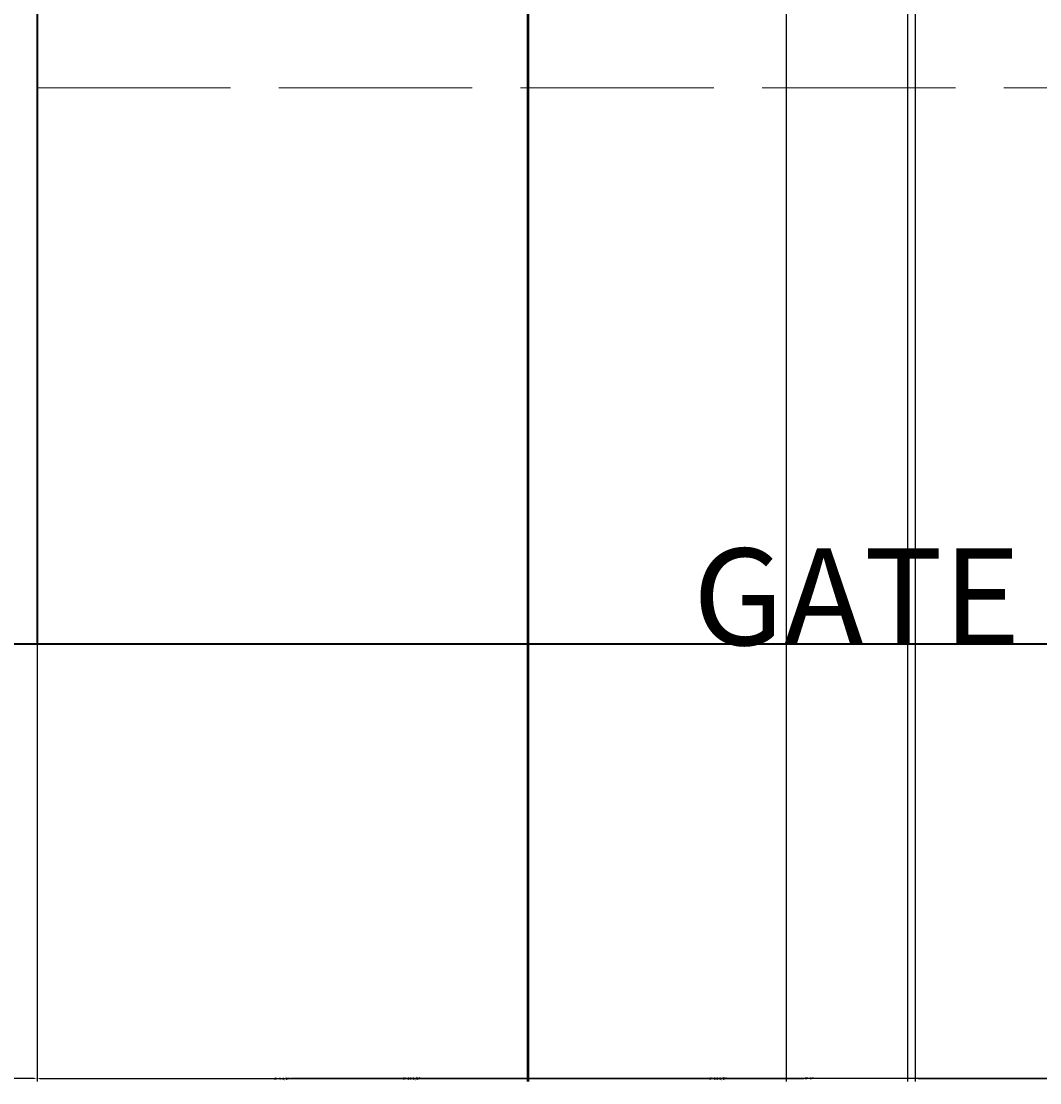
# Model space of a CAD drawing. Units: inches. Extents: x -5 to 330, y -522 to 40.
# Tile 2 of 23: x 32 to 95, y -522 to -457. Entities that reach past the tile are written whole.
import ezdxf

# ---------------------------------------------------------------- set-up
doc = ezdxf.new("R2010")
doc.units = ezdxf.units.IN
doc.header["$MEASUREMENT"] = 0
doc.linetypes.add('ACAD_ISO02W100', pattern=[15, 12, -3])
for name, color, linetype, lineweight in [('A-ANNO-DIMS', 2, 'Continuous', 18), ('A-ANNO-TEXT', 7, 'Continuous', 18), ('A-ROOF-OVHD', 8, 'ACAD_ISO02W100', 18), ('A-SITE-WALL', 7, 'Continuous', 35)]:
    doc.layers.add(name, color=color, linetype=linetype, lineweight=lineweight)
doc.styles.get("Standard").update_dxf_attribs({"font": 'arial.ttf'})
doc.dimstyles.get("Standard").update_dxf_attribs({"dimtxt": 0.18, "dimasz": 0.18, "dimexe": 0.18, "dimexo": 0.0625, "dimgap": 0.09, "dimtad": 0, "dimtih": 1, "dimtoh": 1, "dimdec": 0, "dimzin": 0, "dimdsep": 46, "dimlunit": 3, "dimtxsty": 'Standard', "dimcen": 0.09, "dimadec": 0, "dimazin": 0, "dimtfac": 1, "dimtdec": 0, "dimtofl": 0, "dimtmove": 0, "dimatfit": 3, "dimfxl": 1, "dimtolj": 1, "dimtzin": 0, "dimarcsym": 0})

# ---------------------------------------------------------------- blocks, each defined once
blk = doc.blocks.new('*D39')
at = {"layer": 'A-ANNO-DIMS', "color": 0, "lineweight": -2, "transparency": 16777216}
for p, q in [((32.51, -495.206), (32.51, -522.309)), ((128.361, -495.206), (128.361, -522.309)), ((32.69, -522.129), (80.106, -522.129)), ((128.181, -522.129), (80.765, -522.129))]:
    blk.add_line(p, q, dxfattribs=at)
at = {"layer": 'A-ANNO-DIMS', "color": 0, "transparency": 16777216}
for points in [[(32.69, -522.099), (32.69, -522.159), (32.51, -522.129)], [(128.181, -522.099), (128.181, -522.159), (128.361, -522.129)]]:
    blk.add_solid(points, dxfattribs=at)
at = {"layer": 'Defpoints', "color": 0, "transparency": 16777216}
for p in [(32.51, -495.144), (128.361, -495.144), (128.361, -522.129)]:
    blk.add_point(p, dxfattribs=at)
at = {"layer": 'A-ANNO-DIMS', "color": 0, "transparency": 16777216, "insert": (80.436, -522.129), "char_height": 0.18, "attachment_point": 5}
blk.add_mtext('\\A1;8\'-0"', dxfattribs=at)
blk = doc.blocks.new('*D40')
at = {"layer": 'A-ANNO-DIMS', "color": 0, "lineweight": -2, "transparency": 16777216}
for p, q in [((32.51, -246.706), (32.51, -522.309)), ((79.01, -246.706), (79.01, -522.309)), ((32.69, -522.129), (55.151, -522.129)), ((78.83, -522.129), (56.369, -522.129))]:
    blk.add_line(p, q, dxfattribs=at)
at = {"layer": 'A-ANNO-DIMS', "color": 0, "transparency": 16777216}
for points in [[(32.69, -522.099), (32.69, -522.159), (32.51, -522.129)], [(78.83, -522.099), (78.83, -522.159), (79.01, -522.129)]]:
    blk.add_solid(points, dxfattribs=at)
at = {"layer": 'Defpoints', "color": 0, "transparency": 16777216}
for p in [(32.51, -246.644), (79.01, -246.644), (79.01, -522.129)]:
    blk.add_point(p, dxfattribs=at)
at = {"layer": 'A-ANNO-DIMS', "color": 0, "transparency": 16777216, "insert": (55.76, -522.129), "char_height": 0.18, "attachment_point": 5}
blk.add_mtext('\\A1;3\'-10 1/2"', dxfattribs=at)
blk = doc.blocks.new('*D41')
at = {"layer": 'A-ANNO-DIMS', "color": 0, "lineweight": -2, "transparency": 16777216}
for p, q in [((87.01, -246.706), (87.01, -522.309)), ((129.01, -246.706), (129.01, -522.309)), ((87.19, -522.129), (107.681, -522.129)), ((128.83, -522.129), (108.339, -522.129))]:
    blk.add_line(p, q, dxfattribs=at)
at = {"layer": 'A-ANNO-DIMS', "color": 0, "transparency": 16777216}
for points in [[(87.19, -522.099), (87.19, -522.159), (87.01, -522.129)], [(128.83, -522.099), (128.83, -522.159), (129.01, -522.129)]]:
    blk.add_solid(points, dxfattribs=at)
at = {"layer": 'Defpoints', "color": 0, "transparency": 16777216}
for p in [(87.01, -246.644), (129.01, -246.644), (129.01, -522.129)]:
    blk.add_point(p, dxfattribs=at)
at = {"layer": 'A-ANNO-DIMS', "color": 0, "transparency": 16777216, "insert": (108.01, -522.129), "char_height": 0.18, "attachment_point": 5}
blk.add_mtext('\\A1;3\'-6"', dxfattribs=at)
blk = doc.blocks.new('*D45')
at = {"layer": 'A-ANNO-DIMS', "color": 0, "lineweight": -2, "transparency": 16777216}
for p, q in [((32.51, -417.206), (32.51, -522.309)), ((62.918, -417.206), (62.918, -522.309)), ((32.69, -522.129), (47.173, -522.129)), ((62.738, -522.129), (48.254, -522.129))]:
    blk.add_line(p, q, dxfattribs=at)
at = {"layer": 'A-ANNO-DIMS', "color": 0, "transparency": 16777216}
for points in [[(32.69, -522.099), (32.69, -522.159), (32.51, -522.129)], [(62.738, -522.099), (62.738, -522.159), (62.918, -522.129)]]:
    blk.add_solid(points, dxfattribs=at)
at = {"layer": 'Defpoints', "color": 0, "transparency": 16777216}
for p in [(32.51, -417.144), (62.918, -417.144), (62.918, -522.129)]:
    blk.add_point(p, dxfattribs=at)
at = {"layer": 'A-ANNO-DIMS', "color": 0, "transparency": 16777216, "insert": (47.714, -522.129), "char_height": 0.18, "attachment_point": 5}
blk.add_mtext('\\A1;2\'-6 1/2"', dxfattribs=at)
blk = doc.blocks.new('*D48')
at = {"layer": 'A-ANNO-DIMS', "color": 0, "lineweight": -2, "transparency": 16777216}
for p, q in [((63.01, -416.607), (63.01, -522.309)), ((86.523, -416.607), (86.523, -522.309)), ((63.19, -522.129), (74.166, -522.129)), ((86.343, -522.129), (75.367, -522.129))]:
    blk.add_line(p, q, dxfattribs=at)
at = {"layer": 'A-ANNO-DIMS', "color": 0, "transparency": 16777216}
for points in [[(63.19, -522.099), (63.19, -522.159), (63.01, -522.129)], [(86.343, -522.099), (86.343, -522.159), (86.523, -522.129)]]:
    blk.add_solid(points, dxfattribs=at)
at = {"layer": 'Defpoints', "color": 0, "transparency": 16777216}
for p in [(63.01, -416.544), (86.523, -416.544), (86.523, -522.129)]:
    blk.add_point(p, dxfattribs=at)
at = {"layer": 'A-ANNO-DIMS', "color": 0, "transparency": 16777216, "insert": (74.767, -522.129), "char_height": 0.18, "attachment_point": 5}
blk.add_mtext('\\A1;1\'-11 1/2"', dxfattribs=at)
blk = doc.blocks.new('*D50')
at = {"layer": 'A-ANNO-DIMS', "color": 0, "lineweight": -2, "transparency": 16777216}
for p, q in [((32.51, -417.206), (32.51, -522.309)), ((23.51, -426.206), (23.51, -522.309)), ((23.69, -522.129), (27.681, -522.129)), ((32.33, -522.129), (28.339, -522.129))]:
    blk.add_line(p, q, dxfattribs=at)
at = {"layer": 'A-ANNO-DIMS', "color": 0, "transparency": 16777216}
for points in [[(23.69, -522.099), (23.69, -522.159), (23.51, -522.129)], [(32.33, -522.099), (32.33, -522.159), (32.51, -522.129)]]:
    blk.add_solid(points, dxfattribs=at)
at = {"layer": 'Defpoints', "color": 0, "transparency": 16777216}
for p in [(32.51, -417.144), (23.51, -426.144), (32.51, -522.129)]:
    blk.add_point(p, dxfattribs=at)
at = {"layer": 'A-ANNO-DIMS', "color": 0, "transparency": 16777216, "insert": (28.01, -522.129), "char_height": 0.18, "attachment_point": 5}
blk.add_mtext('\\A1;0\'-9"', dxfattribs=at)

msp = doc.modelspace()

# ---------------------------------------------------------------- linework, layer by layer
at = {"layer": 'A-ROOF-OVHD'}
msp.add_line((32.51, -460.644), (272.01, -460.644), dxfattribs=at)
at = {"layer": 'A-SITE-WALL'}
for p, q in [((32.51, -426.144), (32.51, -495.144)), ((23.51, -495.144), (281.01, -495.144))]:
    msp.add_line(p, q, dxfattribs=at)

# ---------------------------------------------------------------- texts
at = {"layer": 'A-ANNO-TEXT', "insert": (73.21, -489.232), "char_height": 6, "attachment_point": 1}
msp.add_mtext('GATE', dxfattribs=at)

# ---------------------------------------------------------------- dimensions: what is measured, and where the dimension line sits
at = {"layer": 'A-ANNO-DIMS'}
for base, p1, p2, picture, middle in [((79.01, -522.129), (32.51, -246.644), (79.01, -246.644), '*D40', (55.76, -522.129)), ((129.01, -522.129), (87.01, -246.644), (129.01, -246.644), '*D41', (108.01, -522.129)), ((86.523, -522.129), (63.01, -416.544), (86.523, -416.544), '*D48', (74.767, -522.129)), ((32.51, -522.129), (23.51, -426.144), (32.51, -417.144), '*D50', (28.01, -522.129)), ((62.918, -522.129), (32.51, -417.144), (62.918, -417.144), '*D45', (47.714, -522.129)), ((128.361, -522.129), (32.51, -495.144), (128.361, -495.144), '*D39', (80.436, -522.129))]:
    dim = msp.add_linear_dim(base=base, p1=p1, p2=p2, dimstyle='Standard', override={"dimdec": 1, "dimlfac": 1, "dimrnd": 0, "dimzin": 1, "dimdsep": 46, "dimlunit": 4, "dimfrac": 2}, dxfattribs=at)
    dim.commit()
    dim.dimension.update_dxf_attribs({"geometry": picture, "text_midpoint": middle})

doc.saveas('drawing.dxf')
